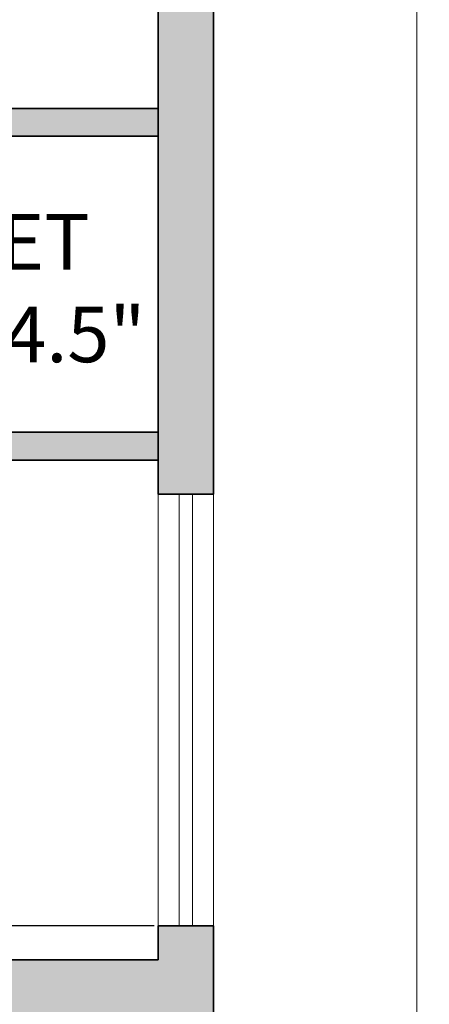
# Model space of a CAD drawing. Units: inches. Extents: x 2696 to 3240, y 1564 to 2310.
# Tile 75 of 76: x 3168 to 3235, y 1982 to 2142. Entities that reach past the tile are written whole.
import ezdxf

# ---------------------------------------------------------------- set-up
doc = ezdxf.new("R2010")
doc.units = ezdxf.units.IN
for name, color, linetype, lineweight in [('A-ANNO-DIMS', 3, 'Continuous', 18), ('A-AREA-IDEN', 7, 'Continuous', 18), ('A-WALL', 7, 'Continuous', 35), ('A-WALL-PATT', 9, 'Continuous', 13), ('WINDOW', 2, 'Continuous', 18)]:
    doc.layers.add(name, color=color, linetype=linetype, lineweight=lineweight)
doc.styles.add('TIMES NEW', font='times.ttf')
doc.styles.add('YQ_DIM', font='SUPEROS.SHX', dxfattribs={"width": 0.8, "bigfont": 'HZDX.SHX'})
doc.dimstyles.new('Siddhuu', dxfattribs={"dimtxt": 6, "dimasz": 2.5, "dimexe": 1.25, "dimexo": 0.625, "dimtad": 1, "dimdec": 1, "dimlunit": 4, "dimtxsty": 'TIMES NEW', "dimcen": 2.5, "dimclrd": 256, "dimclre": 1, "dimclrt": 7, "dimadec": 0, "dimazin": 0, "dimtfac": 1, "dimtdec": 1, "dimtmove": 0, "dimatfit": 3, "dimfxl": 1, "dimtolj": 1, "dimlwd": -1, "dimarcsym": 0})

# ---------------------------------------------------------------- blocks, each defined once
blk = doc.blocks.new('WD_WIN4')
for p, q in [((-0.5, 0.5), (0.5, 0.5)), ((-0.5, 0.12), (0.5, 0.12)), ((-0.5, -0.12), (0.5, -0.12)), ((-0.5, -0.5), (0.5, -0.5))]:
    blk.add_line(p, q)
blk = doc.blocks.new('*D10')
at = {"layer": 'A-ANNO-DIMS', "color": 0, "lineweight": -2, "transparency": 16777216}
for p, q in [((3200.24, 2262.2), (3233.75, 2262.2)), ((3200.24, 1605.2), (3233.75, 1605.2))]:
    blk.add_line(p, q, dxfattribs=at)
at = {"layer": 'A-ANNO-DIMS', "color": 0, "transparency": 16777216}
blk.add_line((3232.5, 2250.2), (3232.5, 1617.2), dxfattribs=at)
for points in [[(3230.5, 2250.2), (3234.5, 2250.2), (3232.5, 2262.2)], [(3230.5, 1617.2), (3234.5, 1617.2), (3232.5, 1605.2)]]:
    blk.add_solid(points, dxfattribs=at)
at = {"layer": 'Defpoints', "color": 0, "transparency": 16777216}
for p in [(3199.61, 2262.2), (3199.61, 1605.2), (3232.5, 1605.2)]:
    blk.add_point(p, dxfattribs=at)
at = {"layer": 'A-ANNO-DIMS', "color": 0, "transparency": 16777216, "insert": (3222.71, 1933.7), "char_height": 18, "attachment_point": 5, "rotation": 90, "style": 'TIMES NEW'}
blk.add_mtext("\\A1;54'", dxfattribs=at)
blk = doc.blocks.new('*D77')
at = {"layer": 'A-ANNO-DIMS', "transparency": 16777216}
for p, q in [((2710.61, 1997.2), (2710.61, 2030.6)), ((2710.61, 1989.2), (2710.61, 1994.7)), ((2710.61, 1986.7), (2710.61, 1984.2))]:
    blk.add_line(p, q, dxfattribs=at)
at = {"layer": 'A-ANNO-DIMS', "color": 1, "lineweight": -2, "transparency": 16777216}
for p, q in [((3189.99, 1994.7), (2709.36, 1994.7)), ((3189.99, 1989.2), (2709.36, 1989.2))]:
    blk.add_line(p, q, dxfattribs=at)
at = {"layer": 'A-ANNO-DIMS', "transparency": 16777216}
for points in [[(2710.19, 1997.2), (2711.03, 1997.2), (2710.61, 1994.7)], [(2710.19, 1986.7), (2711.03, 1986.7), (2710.61, 1989.2)]]:
    blk.add_solid(points, dxfattribs=at)
at = {"layer": 'Defpoints', "color": 0, "transparency": 16777216}
for p in [(2710.61, 1994.7), (3190.61, 1994.7), (3190.61, 1989.2)]:
    blk.add_point(p, dxfattribs=at)
at = {"layer": 'A-ANNO-DIMS', "color": 7, "transparency": 16777216, "insert": (2706.85, 2015.15), "char_height": 6, "attachment_point": 5, "rotation": 90, "style": 'TIMES NEW'}
blk.add_mtext('\\A1;0\'-5 1/2"', dxfattribs=at)

msp = doc.modelspace()

# ---------------------------------------------------------------- hatches: boundary and pattern name
at = {"layer": 'A-WALL-PATT', "transparency": 33554556}
h = msp.add_hatch(color=256, dxfattribs=at)
h.dxf.hatch_style = 1
h.paths.add_polyline_path([(2879.11, 2253.2), (2905.91, 2253.2), (2905.91, 2262.2), (2841.89, 2262.2), (2841.89, 2253.2), (2870.11, 2253.2), (2870.11, 2176.6), (2965.71, 2176.6), (2965.71, 2206.7), (2973.58, 2206.7), (2973.58, 2215.7), (2965.71, 2215.7), (2965.71, 2262.2), (2929.91, 2262.2), (2929.91, 2253.2), (2956.71, 2253.2), (2956.71, 2185.6), (2879.11, 2185.6)])
h.paths.add_polyline_path([(2782.83, 2262.2), (2745.61, 2262.2), (2745.61, 2228.73), (2754.61, 2228.73), (2754.61, 2253.2), (2782.83, 2253.2)])
h.paths.add_polyline_path([(2754.61, 2136.2), (2965.71, 2136.2), (2965.71, 2145.2), (2879.11, 2145.2), (2879.11, 2147.07), (2877.34, 2147.07), (2870.11, 2147.07), (2870.11, 2145.2), (2754.61, 2145.2), (2754.61, 2169.67), (2745.61, 2169.67), (2745.61, 2000.2), (2754.61, 2000.2), (2754.61, 2019.2), (2849.08, 2019.2), (2849.08, 2023.7), (2841.21, 2023.7), (2841.21, 2051.83), (2836.71, 2051.83), (2836.71, 2023.7), (2754.61, 2023.7), (2754.61, 2091.2), (2836.71, 2091.2), (2836.71, 2087.83), (2841.21, 2087.83), (2841.21, 2095.7), (2754.61, 2095.7)])
h.paths.add_polyline_path([(2965.71, 2136.2), (2956.71, 2136.2), (2956.71, 2023.7), (2885.08, 2023.7), (2885.08, 2019.2), (2956.71, 2019.2), (2956.71, 1950.58), (2965.71, 1950.58), (2965.71, 1980.2), (2973.58, 1980.2), (2973.58, 1989.2), (2965.71, 1989.2)])
h.paths.add_polyline_path([(2754.61, 1906.7), (2880.21, 1906.7), (2884.71, 1906.7), (2956.71, 1906.7), (2956.71, 1792.7), (2944.71, 1792.7), (2944.71, 1783.7), (2956.71, 1783.7), (2956.71, 1740.2), (2884.71, 1740.2), (2884.71, 1783.7), (2896.71, 1783.7), (2896.71, 1792.7), (2884.71, 1792.7), (2884.71, 1846.7), (2880.21, 1846.7), (2880.21, 1740.2), (2754.61, 1740.2), (2754.61, 1777.2), (2745.61, 1777.2), (2745.61, 1692.7), (2754.61, 1692.7), (2754.61, 1731.2), (2956.71, 1731.2), (2956.71, 1723.33), (2965.71, 1723.33), (2965.71, 1884.2), (2973.58, 1884.2), (2973.58, 1893.2), (2965.71, 1893.2), (2965.71, 1914.58), (2956.71, 1914.58), (2956.71, 1911.2), (2754.61, 1911.2), (2754.61, 1930.2), (2745.61, 1930.2), (2745.61, 1817.2), (2754.61, 1817.2), (2754.61, 1854.2), (2826.61, 1854.2), (2826.61, 1868.83), (2822.11, 1868.83), (2822.11, 1858.7), (2754.61, 1858.7)])
h.paths.add_polyline_path([(2965.71, 1656.2), (3008.24, 1656.2), (3008.24, 1665.2), (2965.71, 1665.2), (2965.71, 1693.33), (2956.71, 1693.33), (2956.71, 1686.2), (2934.58, 1686.2), (2934.58, 1681.7), (2956.71, 1681.7), (2956.71, 1614.2), (2896.71, 1614.2), (2896.71, 1681.7), (2904.58, 1681.7), (2904.58, 1686.2), (2892.21, 1686.2), (2892.21, 1614.2), (2858.41, 1614.2), (2858.41, 1605.2), (2965.71, 1605.2)])
h.paths.add_polyline_path([(2788.41, 1614.2), (2754.61, 1614.2), (2754.61, 1652.7), (2745.61, 1652.7), (2745.61, 1605.2), (2788.41, 1605.2)])
h.paths.add_polyline_path([(3199.61, 1633.05), (3190.61, 1633.05), (3190.61, 1614.2), (3082.61, 1614.2), (3082.61, 1665.2), (3070.24, 1665.2), (3070.24, 1656.2), (3078.11, 1656.2), (3078.11, 1605.2), (3199.61, 1605.2)])
h.paths.add_polyline_path([(3199.61, 1702.05), (3190.61, 1702.05), (3190.61, 1699.7), (3106.61, 1699.7), (3106.61, 1747.7), (3190.61, 1747.7), (3190.61, 1752.2), (3082.61, 1752.2), (3082.61, 1760.08), (3078.11, 1760.08), (3078.11, 1747.7), (3102.11, 1747.7), (3102.11, 1699.7), (3078.11, 1699.7), (3078.11, 1695.2), (3190.61, 1695.2), (3190.61, 1676.35), (3199.61, 1676.35)])
h.paths.add_polyline_path([(3199.61, 1783.2), (3190.61, 1783.2), (3190.61, 1745.35), (3199.61, 1745.35)])
h.paths.add_polyline_path([(3082.61, 1884.2), (3190.61, 1884.2), (3190.61, 1853.2), (3199.61, 1853.2), (3199.61, 1901.7), (3190.61, 1901.7), (3190.61, 1893.2), (3005.58, 1893.2), (3005.58, 1891.28), (3005.58, 1884.2), (3078.11, 1884.2), (3078.11, 1792.08), (3082.61, 1792.08)])
h.paths.add_polyline_path([(3199.61, 1994.7), (3190.61, 1994.7), (3190.61, 1989.2), (3073.71, 1989.2), (3073.71, 2034.2), (3069.21, 2034.2), (3069.21, 1989.2), (3005.58, 1989.2), (3005.58, 1980.2), (3190.61, 1980.2), (3190.61, 1971.7), (3199.61, 1971.7)])
h.paths.add_polyline_path([(3199.61, 2155.2), (3190.61, 2155.2), (3190.61, 2064.7), (3199.61, 2064.7)])
h.paths.add_polyline_path([(3190.61, 2074.7), (3106.61, 2074.7), (3106.61, 2122.7), (3190.61, 2122.7), (3190.61, 2127.2), (3082.71, 2127.2), (3082.71, 2135.08), (3073.71, 2135.08), (3073.71, 2122.7), (3102.11, 2122.7), (3102.11, 2074.7), (3069.21, 2074.7), (3069.21, 2070.2), (3190.61, 2070.2)])
h.paths.add_polyline_path([(3082.71, 2253.2), (3190.61, 2253.2), (3190.61, 2225.2), (3199.61, 2225.2), (3199.61, 2262.2), (3073.71, 2262.2), (3073.71, 2215.7), (3035.58, 2215.7), (3035.58, 2206.7), (3073.71, 2206.7), (3073.71, 2171.08), (3082.71, 2171.08)])

# ---------------------------------------------------------------- linework, layer by layer
at = {"layer": 'A-WALL'}
for p, q in [((3190.61, 2064.7), (3190.61, 2155.2)), ((3199.61, 2064.7), (3199.61, 2155.2)), ((3082.71, 2127.2), (3190.61, 2127.2)), ((3106.61, 2122.7), (3190.61, 2122.7)), ((3106.61, 2074.7), (3190.61, 2074.7)), ((3069.21, 2070.2), (3190.61, 2070.2)), ((3190.61, 2064.7), (3199.61, 2064.7)), ((3190.61, 1989.2), (3190.61, 1994.7)), ((3190.61, 1994.7), (3199.61, 1994.7)), ((3199.61, 1971.7), (3199.61, 1994.7)), ((3073.71, 1989.2), (3190.61, 1989.2))]:
    msp.add_line(p, q, dxfattribs=at)

# ---------------------------------------------------------------- block references
at = {"layer": 'WINDOW', "xscale": 70, "yscale": 8.999999999999545, "zscale": 70, "rotation": 270}
msp.add_blockref('WD_WIN4', (3195.11, 2029.7), dxfattribs=at)

# ---------------------------------------------------------------- texts
at = {"layer": 'A-AREA-IDEN', "insert": (3138.22, 2110.07), "char_height": 9, "attachment_point": 1, "style": 'YQ_DIM'}
msp.add_mtext_dynamic_manual_height_columns('TOILET\\P5\'X5\'4.5"', width=48.0032, gutter_width=12.5, heights=[0], dxfattribs=at)

# ---------------------------------------------------------------- dimensions: what is measured, and where the dimension line sits
at = {"layer": 'A-ANNO-DIMS'}
dim = msp.add_linear_dim(base=(3232.5, 1605.2), p1=(3199.61, 2262.2), p2=(3199.61, 1605.2), angle=90, text="54'", dimstyle='Siddhuu', override={"dimtxt": 18, "dimasz": 12, "dimclrd": 0, "dimclre": 0, "dimclrt": 0}, dxfattribs=at)
dim.commit()
dim.dimension.update_dxf_attribs({"geometry": '*D10', "text_midpoint": (3222.71, 1933.7)})
dim = msp.add_linear_dim(base=(2710.61, 1994.7), p1=(3190.61, 1989.2), p2=(3190.61, 1994.7), angle=90, dimstyle='Siddhuu', override={"dimdec": 1, "dimlfac": 1, "dimrnd": 0, "dimzin": 1, "dimdsep": 46, "dimlunit": 4, "dimfrac": 2}, dxfattribs=at)
dim.commit()
dim.dimension.update_dxf_attribs({"geometry": '*D77', "text_midpoint": (2706.85, 2015.15)})

doc.saveas('drawing.dxf')
